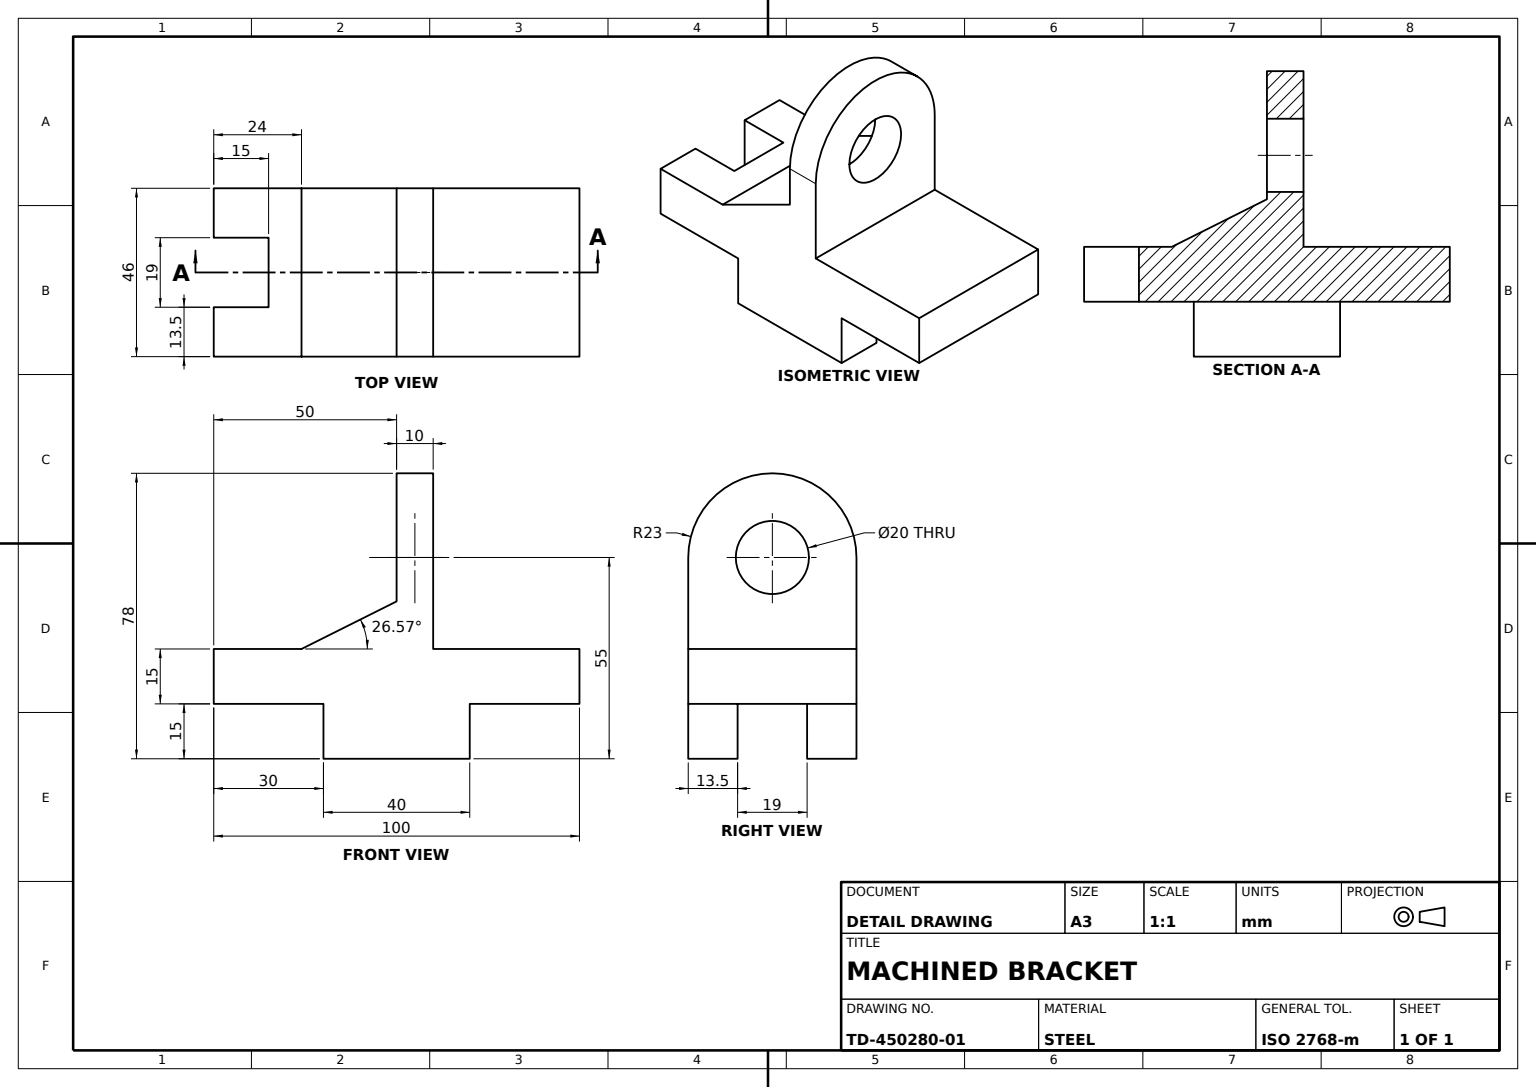
from build123d import *

# Parameters (mm, degrees)
BASE_BODY_DEPTH           = 23
FORK_SLOT_19X15_REACH     = 72.915
FORK_SLOT_SKETCH_W        = 19
FORK_SLOT_SKETCH_H        = 15
CHANNEL_CUT_SKETCH_W      = 19
CHANNEL_CUT_SKETCH_H      = 40
THIN_CHANNEL_CUT_19_DEPTH = 15
LUG_SKETCH_R              = 10
LUG_WITH_BORE_DEPTH       = 10
SUPPORT_RIB_REACH         = 82.206
SUPPORT_RIB_SKETCH_WALL_W = 191.480853336
SUPPORT_RIB_SKETCH_WALL_H = 46


with BuildPart() as part:
    # Base Profile Sketch → Base Body (new, symmetric)
    with BuildSketch(Plane(origin=(0, 0, 0), x_dir=(0, 0, -1), z_dir=(1, 0, 0))):
        Polygon((-60, 0), (40, 0), (40, -15), (10, -15), (10, -30), (-30, -30), (-30, -15), (-60, -15), align=None)
    extrude(amount=BASE_BODY_DEPTH, both=True)

    # Fork Slot Sketch → Fork Slot 19x15 (cut, up to next)
    with BuildSketch(Plane(origin=(0, 0, 0), x_dir=(1, 0, 0), z_dir=(0, 1, 0)), mode=Mode.PRIVATE) as fork_slot_19x15_sk1:
        with Locations((0, -52.5)):
            Rectangle(FORK_SLOT_SKETCH_W, FORK_SLOT_SKETCH_H)
    fork_slot_19x15_tool1 = extrude(fork_slot_19x15_sk1.sketch, amount=-FORK_SLOT_19X15_REACH, mode=Mode.PRIVATE) & part.part
    add(fork_slot_19x15_tool1.solids().sort_by_distance((0, 0, 52.5))[0], mode=Mode.SUBTRACT)

    # Channel Cut Sketch → Thin Channel Cut 19 (cut)
    with BuildSketch(Plane.XZ.offset(30)):
        with Locations((0, 10)):
            Rectangle(CHANNEL_CUT_SKETCH_W, CHANNEL_CUT_SKETCH_H)
    extrude(amount=-THIN_CHANNEL_CUT_19_DEPTH, mode=Mode.SUBTRACT)

    # Lug Sketch → Lug with Bore (add)
    with BuildSketch(Plane.XY):
        with BuildLine():
            Line((23, 25), (23, 0))
            Line((23, 0), (-23, 0))
            Line((-23, 0), (-23, 25))
            ThreePointArc((-23, 25), (0, 48), (23, 25))
        make_face()
        with Locations((0, 25)):
            Circle(LUG_SKETCH_R, mode=Mode.SUBTRACT)
    extrude(amount=LUG_WITH_BORE_DEPTH)

    # Support Rib Sketch wall → Support Rib (add, up to next)
    with BuildSketch(Plane(origin=(0, 6.5, 23), x_dir=(0, -0.4472135955, 0.894427191), z_dir=(0, -0.894427191, -0.4472135955)), mode=Mode.PRIVATE) as support_rib_sk1:
        Rectangle(SUPPORT_RIB_SKETCH_WALL_W, SUPPORT_RIB_SKETCH_WALL_H)
    support_rib_tool1 = extrude(support_rib_sk1.sketch, amount=SUPPORT_RIB_REACH, mode=Mode.PRIVATE) - part.part
    add(support_rib_tool1.solids().sort_by_distance((0, 6.5, 23))[0])


solid = part.part
